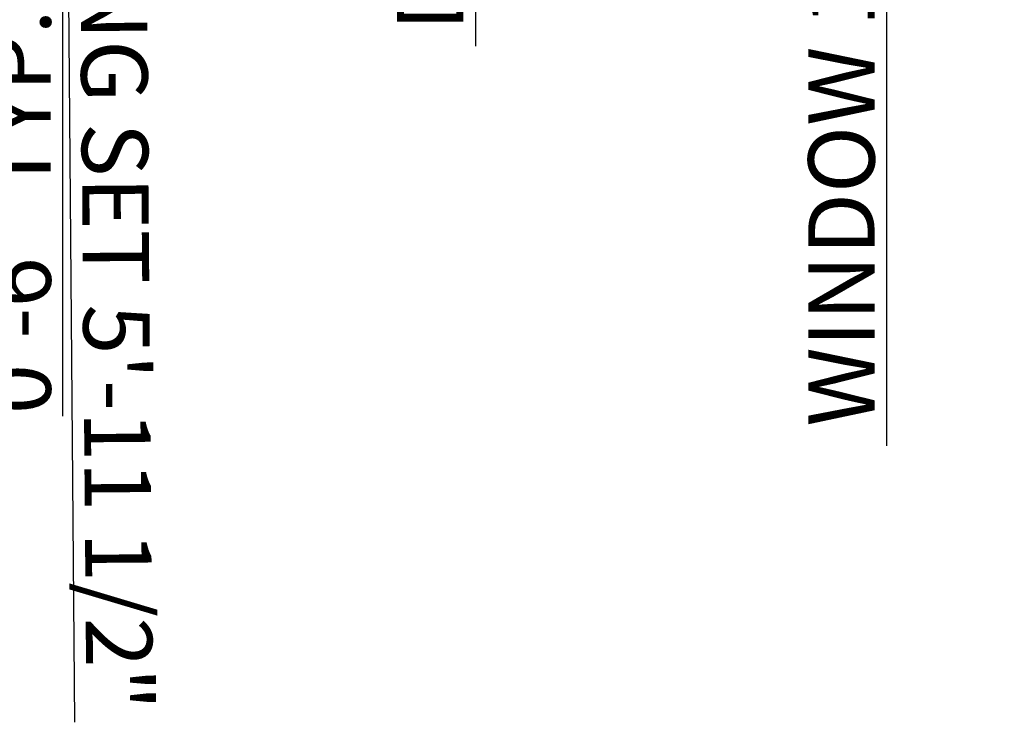
# Model space of a CAD drawing. Units: inches. Extents: x -261 to 409, y 193 to 762.
# Tile 2 of 6: x -35 to 232, y 193 to 384. Entities that reach past the tile are written whole.
import ezdxf

# ---------------------------------------------------------------- set-up
doc = ezdxf.new("R2010")
doc.units = ezdxf.units.IN
doc.layers.add('A-ANNO-DIMS', color=2, linetype='Continuous', lineweight=18)
doc.styles.get("Standard").update_dxf_attribs({"font": 'arial.ttf'})
doc.dimstyles.new('ISO-25', dxfattribs={"dimtxt": 18, "dimasz": 18, "dimexe": 1.25, "dimexo": 0.625, "dimtad": 1, "dimdec": 1, "dimlunit": 3, "dimtxsty": 'Standard', "dimcen": 2.5, "dimadec": 0, "dimazin": 0, "dimtfac": 1, "dimtdec": 1, "dimtmove": 0, "dimatfit": 3, "dimfxl": 1, "dimarcsym": 0})

# ---------------------------------------------------------------- blocks, each defined once
blk = doc.blocks.new('*D11')
at = {"layer": 'A-ANNO-DIMS', "color": 0, "lineweight": -2, "transparency": 16777216}
for p, q in [((88.9, 659.26), (88.9, 677.26)), ((93.68, 641.26), (87.65, 641.26)), ((88.9, 641.26), (88.9, 605.26)), ((93.68, 605.26), (87.65, 605.26)), ((88.9, 587.26), (88.9, 376.77))]:
    blk.add_line(p, q, dxfattribs=at)
at = {"layer": 'A-ANNO-DIMS', "color": 0, "transparency": 16777216}
for points in [[(85.9, 659.26), (91.9, 659.26), (88.9, 641.26)], [(85.9, 587.26), (91.9, 587.26), (88.9, 605.26)]]:
    blk.add_solid(points, dxfattribs=at)
at = {"layer": 'Defpoints', "color": 0, "transparency": 16777216}
for p in [(94.3, 641.26), (88.9, 605.26), (94.3, 605.26)]:
    blk.add_point(p, dxfattribs=at)
at = {"layer": 'A-ANNO-DIMS', "color": 0, "transparency": 16777216, "insert": (78.96, 473.02), "char_height": 18, "attachment_point": 5, "rotation": 90}
blk.add_mtext('DOOR 3\'-0" TYP.', dxfattribs=at)
blk = doc.blocks.new('*D16')
at = {"layer": 'A-ANNO-DIMS', "color": 0, "lineweight": -2, "transparency": 16777216}
for p, q in [((-23.2, 447.26), (-23.2, 465.26)), ((-14.82, 429.26), (-24.45, 429.26)), ((-23.2, 429.26), (-23.2, 423.26)), ((-14.82, 423.26), (-24.45, 423.26)), ((-23.2, 405.26), (-23.2, 276.29))]:
    blk.add_line(p, q, dxfattribs=at)
at = {"layer": 'A-ANNO-DIMS', "color": 0, "transparency": 16777216}
for points in [[(-26.2, 447.26), (-20.2, 447.26), (-23.2, 429.26)], [(-26.2, 405.26), (-20.2, 405.26), (-23.2, 423.26)]]:
    blk.add_solid(points, dxfattribs=at)
at = {"layer": 'Defpoints', "color": 0, "transparency": 16777216}
for p in [(-14.2, 429.26), (-23.2, 423.26), (-14.2, 423.26)]:
    blk.add_point(p, dxfattribs=at)
at = {"layer": 'A-ANNO-DIMS', "color": 0, "transparency": 16777216, "insert": (-33.01, 331.78), "char_height": 18, "attachment_point": 5, "rotation": 90}
blk.add_mtext('0\'-6" TYP.', dxfattribs=at)
blk = doc.blocks.new('*D17')
at = {"layer": 'A-ANNO-DIMS', "color": 0, "lineweight": -2, "transparency": 16777216}
for p, q in [((200.5, 563.26), (200.5, 581.26)), ((201.68, 545.26), (199.25, 545.26)), ((200.5, 545.26), (200.5, 533.26)), ((201.68, 533.26), (199.25, 533.26)), ((200.5, 515.26), (200.5, 268.24))]:
    blk.add_line(p, q, dxfattribs=at)
at = {"layer": 'A-ANNO-DIMS', "color": 0, "transparency": 16777216}
for points in [[(197.5, 563.26), (203.5, 563.26), (200.5, 545.26)], [(197.5, 515.26), (203.5, 515.26), (200.5, 533.26)]]:
    blk.add_solid(points, dxfattribs=at)
at = {"layer": 'Defpoints', "color": 0, "transparency": 16777216}
for p in [(202.3, 545.26), (200.5, 533.26), (202.3, 533.26)]:
    blk.add_point(p, dxfattribs=at)
at = {"layer": 'A-ANNO-DIMS', "color": 0, "transparency": 16777216, "insert": (190.56, 382.75), "char_height": 18, "attachment_point": 5, "rotation": 90}
blk.add_mtext('WINDOW 1\'-0" TYP.', dxfattribs=at)
blk = doc.blocks.new('*D21')
at = {"layer": 'A-ANNO-DIMS', "color": 0, "lineweight": -2, "transparency": 16777216}
for p, q in [((-12.58, 537.97), (-23.96, 537.88)), ((-22.56, 519.89), (-22.27, 484.23)), ((-12, 466.31), (-23.38, 466.22)), ((-22.13, 466.23), (-19.92, 193.22))]:
    blk.add_line(p, q, dxfattribs=at)
at = {"layer": 'A-ANNO-DIMS', "color": 0, "transparency": 16777216}
for points in [[(-19.56, 519.92), (-25.56, 519.87), (-22.71, 537.89)], [(-19.27, 484.25), (-25.27, 484.2), (-22.13, 466.23)]]:
    blk.add_solid(points, dxfattribs=at)
at = {"layer": 'Defpoints', "color": 0, "transparency": 16777216}
for p in [(-11.96, 537.98), (-22.13, 466.23), (-11.38, 466.31)]:
    blk.add_point(p, dxfattribs=at)
at = {"layer": 'A-ANNO-DIMS', "color": 0, "transparency": 16777216, "insert": (-11.02, 320.8), "char_height": 18, "attachment_point": 5, "rotation": 270.4625}
blk.add_mtext('DINING SET 5\'-11 1/2"', dxfattribs=at)

msp = doc.modelspace()

# ---------------------------------------------------------------- dimensions: what is measured, and where the dimension line sits
at = {"layer": 'A-ANNO-DIMS'}
for base, p1, p2, angle, text, picture, middle in [((88.9, 605.26), (94.3, 641.26), (94.3, 605.26), 270, 'DOOR <> TYP.', '*D11', (78.96, 473.02)), ((200.5, 533.26), (202.3, 545.26), (202.3, 533.26), 270, 'WINDOW <> TYP.', '*D17', (190.56, 382.75)), ((-22.13, 466.23), (-11.96, 537.98), (-11.38, 466.31), 270.4625, 'DINING SET <>', '*D21', (-11.02, 320.8)), ((-23.2, 423.26), (-14.2, 429.26), (-14.2, 423.26), 270, '<> TYP.', '*D16', (-33.01, 331.78))]:
    dim = msp.add_linear_dim(base=base, p1=p1, p2=p2, angle=angle, text=text, dimstyle='ISO-25', override={"dimdec": 1, "dimlfac": 1, "dimrnd": 0, "dimzin": 1, "dimdsep": 46, "dimlunit": 4, "dimfrac": 2}, dxfattribs=at)
    dim.commit()
    dim.dimension.update_dxf_attribs({"geometry": picture, "text_midpoint": middle})

doc.saveas('drawing.dxf')
